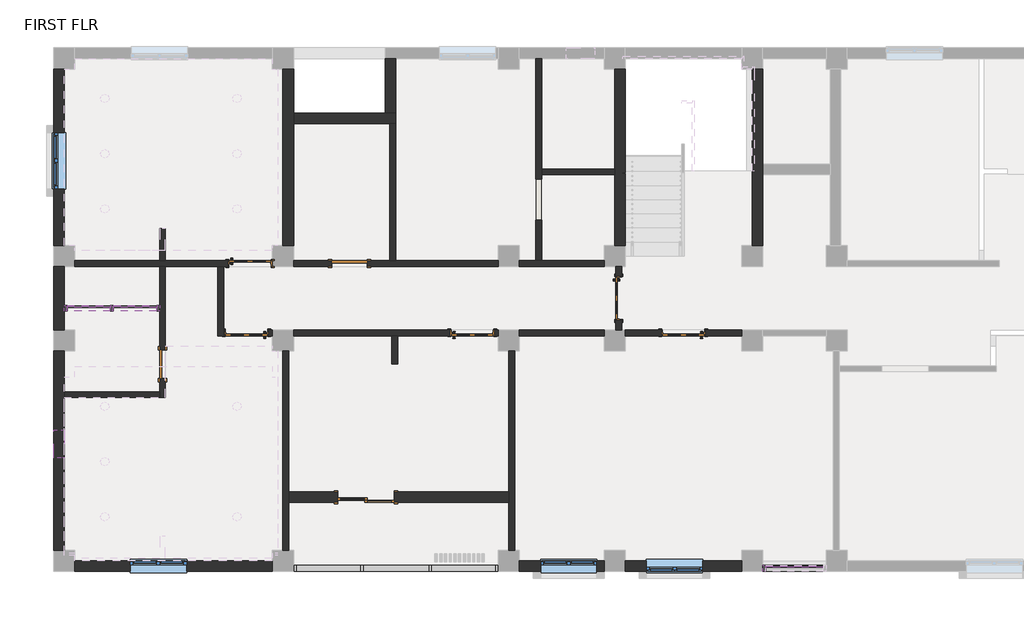
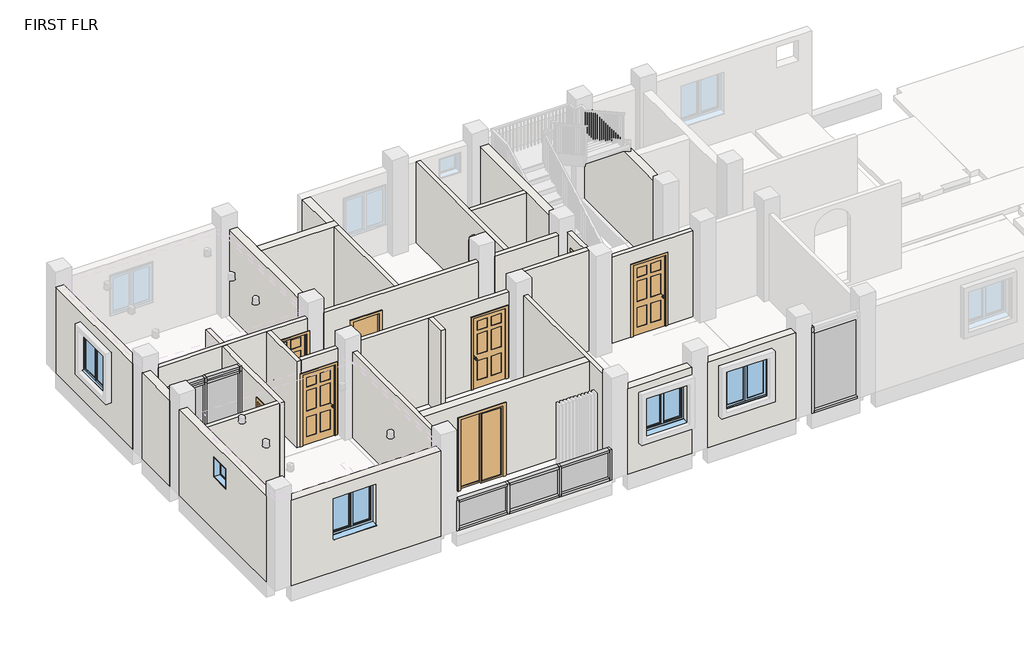
# One storey, part 1 of 5: 29 walls, 25 members, 9 plates, 8 doors, 5 windows.
"""IFC4 building model written with IfcOpenShell, lengths in millimetres."""

from ifc_helpers import new_model, si_unit, point, frame, origin, place, context, project, spatial, polyline, ellipse_curve, trimmed, outline, extrude, faceted_brep, transform, mapped, element, save
from ifc_brep_helpers import plane_surface, extruded_surface, advanced_brep
from components import door_double_sliding_4436dcad, door_c610b25b, door_03e3dfb5, single_flush_2_x_7_bath_room_door_025d1c86, door_e00f436c, member_f0fea5a5, member_f6f0dfdd, member_ee409385, member_876f8f00, member_2b4cd6f1, member_0dc43c0c, member_51239652, member_c58de4df, member_410c6227, member_73c23c35, member_71eb4692, system_panel_glazed_e8343dfa, system_panel_glazed_58efc156, system_panel_glazed_69a0d9e9, system_panel_glazed_27716cba, system_panel_glazed_e6f1e35b, system_panel_glazed_aa2ae1c5, window_80340324, w2_0001_4_x_4_window_9dec5fc7

model = new_model("IFC4")

# Units and contexts
model_context = context("Model", 3, world=origin())
ifc_project = project(units=[si_unit("LENGTHUNIT", "METRE", prefix="MILLI")], contexts=[model_context])

# Site, building, storey
site = spatial("IfcSite", under=ifc_project)
building = spatial("IfcBuilding", under=site)
storey = spatial("IfcBuildingStorey", under=building, Name="FIRST FLR", Elevation=3352.8)

# Doors
placement = place(None, origin())
door_double_sliding_shape = door_double_sliding_4436dcad(model_context)
element("IfcDoor", 1, ObjectType="Door-Double-Sliding", at=placement, inside=storey, context=model_context, shape_type="MappedRepresentation", body=[
    mapped(door_double_sliding_shape, transform((-8630.2456086, -9389.2679047, 3352.8), x_axis=(-1.0, 0.0, 0.0), y_axis=(0.0, -1.0, 0.0), z_axis=(0.0, 0.0, 1.0))),
])
door_shape = door_c610b25b(model_context)
element("IfcDoor", 2, ObjectType="Door-Interior-Single-6_Panel-Wood : 36\" x 84\"", at=placement, inside=storey, context=model_context, shape_type="MappedRepresentation", body=[
    mapped(door_shape, transform((-6331.5456086, -5967.8544704, 3352.8), x_axis=(1.0, 0.0, 0.0), y_axis=(0.0, 1.0, 0.0), z_axis=(0.0, 0.0, 1.0))),
])
element("IfcDoor", 3, ObjectType="Door-Interior-Single-6_Panel-Wood : 36\" x 84\"", at=placement, inside=storey, context=model_context, shape_type="MappedRepresentation", body=[
    mapped(door_shape, transform((-3172.4206086, -5215.3794704, 3352.8), x_axis=(0.0, -1.0, 0.0), y_axis=(1.0, 0.0, 0.0), z_axis=(0.0, 0.0, 1.0))),
])
door_2_shape = door_03e3dfb5(model_context)
element("IfcDoor", 4, ObjectType="Door-Interior-Single-6_Panel-Wood : 36\" x 84\"", at=placement, inside=storey, context=model_context, shape_type="MappedRepresentation", body=[
    mapped(door_2_shape, transform((-11207.742897, -5967.8544704, 3352.8), x_axis=(-1.0, 0.0, 0.0), y_axis=(0.0, -1.0, 0.0), z_axis=(0.0, 0.0, 1.0))),
])
element("IfcDoor", 5, ObjectType="Door-Interior-Single-6_Panel-Wood : 36\" x 84\"", at=placement, inside=storey, context=model_context, shape_type="MappedRepresentation", body=[
    mapped(door_2_shape, transform((-11132.1456086, -4462.9044704, 3352.8), x_axis=(1.0, 0.0, 0.0), y_axis=(0.0, 1.0, 0.0), z_axis=(0.0, 0.0, 1.0))),
])
element("IfcDoor", 6, ObjectType="Door-Interior-Single-6_Panel-Wood : 36\" x 84\"", at=placement, inside=storey, context=model_context, shape_type="MappedRepresentation", body=[
    mapped(door_2_shape, transform((-1773.9769742, -5967.8544704, 3352.8), x_axis=(-1.0, 0.0, 0.0), y_axis=(0.0, -1.0, 0.0), z_axis=(0.0, 0.0, 1.0))),
])
single_flush_2_x_7_bath_room_door_shape = single_flush_2_x_7_bath_room_door_025d1c86(model_context)
element("IfcDoor", 7, ObjectType="Single-Flush : 2' X 7' BATH ROOM DOOR", at=placement, inside=storey, context=model_context, shape_type="MappedRepresentation", body=[
    mapped(single_flush_2_x_7_bath_room_door_shape, transform((-13023.2401855, -6639.2659448, 3352.8), x_axis=(0.0, 1.0, 0.0), y_axis=(-1.0, 0.0, 0.0), z_axis=(0.0, 0.0, 1.0))),
])
door_3_shape = door_e00f436c(model_context)
element("IfcDoor", 8, ObjectType="Single-Flush : bathroom 2'6\" door", at=placement, inside=storey, context=model_context, shape_type="MappedRepresentation", body=[
    mapped(door_3_shape, transform((-8985.8456086, -4466.0794704, 3352.8), x_axis=(-1.0, 0.0, 0.0), y_axis=(0.0, -1.0, 0.0), z_axis=(0.0, 0.0, 1.0))),
])

# Members
member_shape = member_f0fea5a5(model_context)
element("IfcMember", 9, ObjectType="Rectangular Mullion : 2.5\" x 5\" rectangular", at=placement, inside=storey, context=model_context, shape_type="MappedRepresentation", body=[
    mapped(member_shape, transform((-14116.042897, -5431.2794704, 3352.8), x_axis=(1.0, 0.0, 0.0), y_axis=(0.0, -1.0, 0.0), z_axis=(0.0, 0.0, -1.0))),
])
member_2_shape = member_f6f0dfdd(model_context)
element("IfcMember", 10, ObjectType="Rectangular Mullion : 2.5\" x 5\" rectangular", at=placement, inside=storey, context=model_context, shape_type="MappedRepresentation", body=[
    mapped(member_2_shape, transform((-14116.042897, -5431.2794704, 5791.2), x_axis=(1.0, 0.0, 0.0), y_axis=(0.0, -1.0, 0.0), z_axis=(0.0, 0.0, -1.0))),
])
member_3_shape = member_ee409385(model_context)
element("IfcMember", 11, ObjectType="Rectangular Mullion : 2.5\" x 5\" rectangular", at=placement, inside=storey, context=model_context, shape_type="MappedRepresentation", body=[
    mapped(member_3_shape, transform((-13086.7401855, -5431.2794704, 3352.8), x_axis=(1.0, 0.0, 0.0), y_axis=(0.0, -1.0, 0.0), z_axis=(0.0, 0.0, -1.0))),
])
member_4_shape = member_876f8f00(model_context)
element("IfcMember", 12, ObjectType="Rectangular Mullion : 2.5\" x 5\" rectangular", at=placement, inside=storey, context=model_context, shape_type="MappedRepresentation", body=[
    mapped(member_4_shape, transform((-15145.3456086, -5431.2794704, 5943.6), x_axis=(-1.0, 0.0, 0.0), y_axis=(0.0, -1.0, 0.0), z_axis=(0.0, 0.0, 1.0))),
])
element("IfcMember", 13, ObjectType="Rectangular Mullion : 2.5\" x 5\" rectangular", at=placement, inside=storey, context=model_context, shape_type="MappedRepresentation", body=[
    mapped(member_4_shape, transform((-61.2083398, -11052.9679047, 5943.6), x_axis=(-1.0, 0.0, 0.0), y_axis=(0.0, -1.0, 0.0), z_axis=(0.0, 0.0, 1.0))),
])
element("IfcMember", 14, ObjectType="Rectangular Mullion : 2.5\" x 5\" rectangular", at=placement, inside=storey, context=model_context, shape_type="MappedRepresentation", body=[
    mapped(member_4_shape, transform((-13086.7401855, -5431.2794704, 5791.2), x_axis=(1.0, 0.0, 0.0), y_axis=(0.0, -1.0, 0.0), z_axis=(0.0, 0.0, -1.0))),
])
element("IfcMember", 15, ObjectType="Rectangular Mullion : 2.5\" x 5\" rectangular", at=placement, inside=storey, context=model_context, shape_type="MappedRepresentation", body=[
    mapped(member_3_shape, transform((-15145.3456086, -5431.2794704, 5791.2), x_axis=(-1.0, 0.0, 0.0), y_axis=(0.0, -1.0, 0.0), z_axis=(0.0, 0.0, 1.0))),
])
element("IfcMember", 16, ObjectType="Rectangular Mullion : 2.5\" x 5\" rectangular", at=placement, inside=storey, context=model_context, shape_type="MappedRepresentation", body=[
    mapped(member_3_shape, transform((-61.2083398, -11052.9679047, 5791.2), x_axis=(-1.0, 0.0, 0.0), y_axis=(0.0, -1.0, 0.0), z_axis=(0.0, 0.0, 1.0))),
])
member_5_shape = member_2b4cd6f1(model_context)
element("IfcMember", 17, ObjectType="Rectangular Mullion : 2.5\" x 5\" rectangular", at=placement, inside=storey, context=model_context, shape_type="MappedRepresentation", body=[
    mapped(member_5_shape, transform((-5836.2456086, -11052.9679047, 4267.2), x_axis=(0.0, 0.0, 1.0), y_axis=(0.0, -1.0, 0.0), z_axis=(1.0, 0.0, 0.0))),
])
element("IfcMember", 18, ObjectType="Rectangular Mullion : 2.5\" x 5\" rectangular", at=placement, inside=storey, context=model_context, shape_type="MappedRepresentation", body=[
    mapped(member_5_shape, transform((-8750.8956085, -11052.9679047, 4267.2), x_axis=(0.0, 0.0, 1.0), y_axis=(0.0, -1.0, 0.0), z_axis=(1.0, 0.0, 0.0))),
])
element("IfcMember", 19, ObjectType="Rectangular Mullion : 2.5\" x 5\" rectangular", at=placement, inside=storey, context=model_context, shape_type="MappedRepresentation", body=[
    mapped(member_5_shape, transform((-10128.8456086, -11052.9679047, 3352.8), x_axis=(0.0, 0.0, -1.0), y_axis=(0.0, -1.0, 0.0), z_axis=(-1.0, 0.0, 0.0))),
])
element("IfcMember", 20, ObjectType="Rectangular Mullion : 2.5\" x 5\" rectangular", at=placement, inside=storey, context=model_context, shape_type="MappedRepresentation", body=[
    mapped(member_5_shape, transform((-7214.1956087, -11052.9679047, 3352.8), x_axis=(0.0, 0.0, -1.0), y_axis=(0.0, -1.0, 0.0), z_axis=(-1.0, 0.0, 0.0))),
])
member_6_shape = member_0dc43c0c(model_context)
element("IfcMember", 21, ObjectType="Rectangular Mullion : 2.5\" x 5\" rectangular", at=placement, inside=storey, context=model_context, shape_type="MappedRepresentation", body=[
    mapped(member_6_shape, transform((-7277.6956087, -11052.9679047, 4267.2), x_axis=(0.0, 0.0, 1.0), y_axis=(0.0, -1.0, 0.0), z_axis=(1.0, 0.0, 0.0))),
])
element("IfcMember", 22, ObjectType="Rectangular Mullion : 2.5\" x 5\" rectangular", at=placement, inside=storey, context=model_context, shape_type="MappedRepresentation", body=[
    mapped(member_6_shape, transform((-8687.3956085, -11052.9679047, 3352.8), x_axis=(0.0, 0.0, -1.0), y_axis=(0.0, -1.0, 0.0), z_axis=(-1.0, 0.0, 0.0))),
])
member_7_shape = member_51239652(model_context)
element("IfcMember", 23, ObjectType="Rectangular Mullion : 2.5\" x 5\" rectangular", at=placement, inside=storey, context=model_context, shape_type="MappedRepresentation", body=[
    mapped(member_7_shape, transform((-13150.2401855, -5431.2794704, 5943.6), x_axis=(0.0, 0.0, 1.0), y_axis=(0.0, -1.0, 0.0), z_axis=(1.0, 0.0, 0.0))),
])
element("IfcMember", 24, ObjectType="Rectangular Mullion : 2.5\" x 5\" rectangular", at=placement, inside=storey, context=model_context, shape_type="MappedRepresentation", body=[
    mapped(member_7_shape, transform((-14147.792897, -5431.2794704, 5943.6), x_axis=(0.0, 0.0, 1.0), y_axis=(0.0, -1.0, 0.0), z_axis=(1.0, 0.0, 0.0))),
])
element("IfcMember", 25, ObjectType="Rectangular Mullion : 2.5\" x 5\" rectangular", at=placement, inside=storey, context=model_context, shape_type="MappedRepresentation", body=[
    mapped(member_7_shape, transform((-15081.8456086, -5431.2794704, 3352.8), x_axis=(0.0, 0.0, -1.0), y_axis=(0.0, -1.0, 0.0), z_axis=(-1.0, 0.0, 0.0))),
])
element("IfcMember", 26, ObjectType="Rectangular Mullion : 2.5\" x 5\" rectangular", at=placement, inside=storey, context=model_context, shape_type="MappedRepresentation", body=[
    mapped(member_7_shape, transform((-14084.292897, -5431.2794704, 3352.8), x_axis=(0.0, 0.0, -1.0), y_axis=(0.0, -1.0, 0.0), z_axis=(-1.0, 0.0, 0.0))),
])
member_8_shape = member_c58de4df(model_context)
element("IfcMember", 27, ObjectType="Rectangular Mullion : 2.5\" x 5\" rectangular", at=placement, inside=storey, context=model_context, shape_type="MappedRepresentation", body=[
    mapped(member_8_shape, transform((-14147.792897, -5431.2794704, 5791.2), x_axis=(0.0, 0.0, 1.0), y_axis=(0.0, -1.0, 0.0), z_axis=(1.0, 0.0, 0.0))),
])
element("IfcMember", 28, ObjectType="Rectangular Mullion : 2.5\" x 5\" rectangular", at=placement, inside=storey, context=model_context, shape_type="MappedRepresentation", body=[
    mapped(member_8_shape, transform((-13150.2401855, -5431.2794704, 5791.2), x_axis=(0.0, 0.0, 1.0), y_axis=(0.0, -1.0, 0.0), z_axis=(1.0, 0.0, 0.0))),
])
member_9_shape = member_410c6227(model_context)
element("IfcMember", 29, ObjectType="Rectangular Mullion : 2.5\" x 5\" rectangular", at=placement, inside=storey, context=model_context, shape_type="MappedRepresentation", body=[
    mapped(member_9_shape, transform((-8719.1456085, -11052.9679047, 3352.8), x_axis=(1.0, 0.0, 0.0), y_axis=(0.0, -1.0, 0.0), z_axis=(0.0, 0.0, -1.0))),
])
element("IfcMember", 30, ObjectType="Rectangular Mullion : 2.5\" x 5\" rectangular", at=placement, inside=storey, context=model_context, shape_type="MappedRepresentation", body=[
    mapped(member_9_shape, transform((-7245.9456087, -11052.9679047, 3352.8), x_axis=(1.0, 0.0, 0.0), y_axis=(0.0, -1.0, 0.0), z_axis=(0.0, 0.0, -1.0))),
])
member_10_shape = member_73c23c35(model_context)
element("IfcMember", 31, ObjectType="Rectangular Mullion : 2.5\" x 5\" rectangular", at=placement, inside=storey, context=model_context, shape_type="MappedRepresentation", body=[
    mapped(member_10_shape, transform((-5772.7456086, -11052.9679047, 3352.8), x_axis=(1.0, 0.0, 0.0), y_axis=(0.0, -1.0, 0.0), z_axis=(0.0, 0.0, -1.0))),
])
element("IfcMember", 32, ObjectType="Rectangular Mullion : 2.5\" x 5\" rectangular", at=placement, inside=storey, context=model_context, shape_type="MappedRepresentation", body=[
    mapped(member_10_shape, transform((-10192.3456086, -11052.9679047, 4267.2), x_axis=(-1.0, 0.0, 0.0), y_axis=(0.0, -1.0, 0.0), z_axis=(0.0, 0.0, 1.0))),
])
member_11_shape = member_71eb4692(model_context)
element("IfcMember", 33, ObjectType="Rectangular Mullion : 2.5\" x 5\" rectangular", at=placement, inside=storey, context=model_context, shape_type="MappedRepresentation", body=[
    mapped(member_11_shape, transform((2.2916602, -11052.9679047, 3352.8), x_axis=(0.0, 0.0, -1.0), y_axis=(0.0, -1.0, 0.0), z_axis=(-1.0, 0.0, 0.0))),
])

# Plates
system_panel_glazed_shape = system_panel_glazed_e8343dfa(model_context)
element("IfcPlate", 34, ObjectType="System Panel : Glazed", at=placement, inside=storey, context=model_context, shape_type="MappedRepresentation", body=[
    mapped(system_panel_glazed_shape, transform((-14614.8192528, -5431.2794704, 3416.3), x_axis=(1.0, 0.0, 0.0), y_axis=(0.0, 1.0, 0.0), z_axis=(0.0, 0.0, 1.0))),
])
element("IfcPlate", 35, ObjectType="System Panel : Glazed", at=placement, inside=storey, context=model_context, shape_type="MappedRepresentation", body=[
    mapped(system_panel_glazed_shape, transform((-13617.2665413, -5431.2794704, 3416.3), x_axis=(1.0, 0.0, 0.0), y_axis=(0.0, 1.0, 0.0), z_axis=(0.0, 0.0, 1.0))),
])
system_panel_glazed_2_shape = system_panel_glazed_58efc156(model_context)
element("IfcPlate", 36, ObjectType="System Panel : Glazed", at=placement, inside=storey, context=model_context, shape_type="MappedRepresentation", body=[
    mapped(system_panel_glazed_2_shape, transform((-14614.8192528, -5431.2794704, 5822.95), x_axis=(1.0, 0.0, 0.0), y_axis=(0.0, 1.0, 0.0), z_axis=(0.0, 0.0, 1.0))),
])
element("IfcPlate", 37, ObjectType="System Panel : Glazed", at=placement, inside=storey, context=model_context, shape_type="MappedRepresentation", body=[
    mapped(system_panel_glazed_2_shape, transform((-13617.2665413, -5431.2794704, 5822.95), x_axis=(1.0, 0.0, 0.0), y_axis=(0.0, 1.0, 0.0), z_axis=(0.0, 0.0, 1.0))),
])
system_panel_glazed_3_shape = system_panel_glazed_69a0d9e9(model_context)
element("IfcPlate", 38, ObjectType="System Panel : Glazed", at=placement, inside=storey, context=model_context, shape_type="MappedRepresentation", body=[
    mapped(system_panel_glazed_3_shape, transform((-9439.8706086, -11052.9679047, 3416.3), x_axis=(1.0, 0.0, 0.0), y_axis=(0.0, 1.0, 0.0), z_axis=(0.0, 0.0, 1.0))),
])
element("IfcPlate", 39, ObjectType="System Panel : Glazed", at=placement, inside=storey, context=model_context, shape_type="MappedRepresentation", body=[
    mapped(system_panel_glazed_3_shape, transform((-6525.2206087, -11052.9679047, 3416.3), x_axis=(1.0, 0.0, 0.0), y_axis=(0.0, 1.0, 0.0), z_axis=(0.0, 0.0, 1.0))),
])
system_panel_glazed_4_shape = system_panel_glazed_27716cba(model_context)
element("IfcPlate", 40, ObjectType="System Panel : Glazed", at=placement, inside=storey, context=model_context, shape_type="MappedRepresentation", body=[
    mapped(system_panel_glazed_4_shape, transform((-7982.5456086, -11052.9679047, 3416.3), x_axis=(1.0, 0.0, 0.0), y_axis=(0.0, 1.0, 0.0), z_axis=(0.0, 0.0, 1.0))),
])
system_panel_glazed_5_shape = system_panel_glazed_e6f1e35b(model_context)
element("IfcPlate", 41, ObjectType="System Panel : Glazed", at=placement, inside=storey, context=model_context, shape_type="MappedRepresentation", body=[
    mapped(system_panel_glazed_5_shape, transform((624.5916602, -11052.9679047, 3416.3), x_axis=(1.0, 0.0, 0.0), y_axis=(0.0, 1.0, 0.0), z_axis=(0.0, 0.0, 1.0))),
])
system_panel_glazed_6_shape = system_panel_glazed_aa2ae1c5(model_context)
element("IfcPlate", 42, ObjectType="System Panel : Glazed", at=placement, inside=storey, context=model_context, shape_type="MappedRepresentation", body=[
    mapped(system_panel_glazed_6_shape, transform((624.5916602, -11052.9679047, 5822.95), x_axis=(1.0, 0.0, 0.0), y_axis=(0.0, 1.0, 0.0), z_axis=(0.0, 0.0, 1.0))),
])

# Walls
element("IfcWall", 43, ObjectType="EXTERIOR WALL 9\"", at=placement, inside=storey, context=model_context, shape_type="SweptSolid", body=[
    extrude(outline(polyline([(3352.8, -14916.7456086), (3352.8, -10649.5456086), (5943.6, -10649.5456086), (5943.6, -14916.7456086), (3352.8, -14916.7456086)]), holes=[polyline([(4352.8, -12503.7456086), (4352.8, -13722.9456086), (5572.0, -13722.9456086), (5572.0, -12503.7456086), (4352.8, -12503.7456086)])]), frame((0.0, -11116.4679047, 0.0), z_axis=(0.0, 1.0, 0.0), x_axis=(0.0, 0.0, 1.0)), (0.0, 0.0, 1.0), 228.6),
])
element("IfcWall", 44, ObjectType="EXTERIOR WALL 9\"", at=placement, inside=storey, context=model_context, shape_type="SweptSolid", body=[
    extrude(outline(polyline([(3352.8, -5315.5456086), (3352.8, -3486.7456086), (5943.6, -3486.7456086), (5943.6, -5315.5456086), (3352.8, -5315.5456086)]), holes=[polyline([(4352.8, -3639.1456086), (4352.8, -4858.3456086), (5572.0, -4858.3456086), (5572.0, -3639.1456086), (4352.8, -3639.1456086)])]), frame((0.0, -11116.4679047, 0.0), z_axis=(0.0, 1.0, 0.0), x_axis=(0.0, 0.0, 1.0)), (0.0, 0.0, 1.0), 228.6),
])
element("IfcWall", 45, ObjectType="EXTERIOR WALL 9\"", at=placement, inside=storey, context=model_context, shape_type="SweptSolid", body=[
    extrude(outline(polyline([(3352.8, -3029.5456086), (3352.8, -518.4083398), (5943.6, -518.4083398), (5943.6, -3029.5456086), (3352.8, -3029.5456086)]), holes=[polyline([(4352.8, -2572.3456086), (5572.0, -2572.3456086), (5572.0, -1353.1456086), (4352.8, -1353.1456086), (4352.8, -2572.3456086)])]), frame((0.0, -11116.4679047, 0.0), z_axis=(0.0, 1.0, 0.0), x_axis=(0.0, 0.0, 1.0)), (0.0, 0.0, 1.0), 228.6),
])
element("IfcWall", 46, ObjectType="EXTERIOR WALL 9\"", at=placement, inside=storey, context=model_context, shape_type="Brep", body=[
    faceted_brep([(-15145.3456086, -10659.2679047, 3352.8), (-15145.3456086, -7363.1659448, 3352.8), (-15145.3456086, -7236.1659448, 3352.8), (-15145.3456086, -6358.3794704, 3352.8), (-15145.3456086, -6358.3794704, 5943.6), (-15145.3456086, -7236.1659448, 5943.6), (-15145.3456086, -7363.1659448, 5943.6), (-15145.3456086, -10659.2679047, 5943.6), (-15145.3456086, -8671.2659448, 5559.8263913), (-15145.3456086, -8061.6659448, 5559.8263913), (-15145.3456086, -8061.6659448, 4950.2263913), (-15145.3456086, -8671.2659448, 4950.2263913), (-15373.9456086, -10659.2679047, 3352.8), (-15373.9456086, -10659.2679047, 5943.6), (-15373.9456086, -6358.3794704, 5943.6), (-15373.9456086, -6358.3794704, 3352.8), (-15373.9456086, -8671.2659448, 5559.8263913), (-15373.9456086, -8671.2659448, 4950.2263913), (-15373.9456086, -8061.6659448, 4950.2263913), (-15373.9456086, -8061.6659448, 5559.8263913)], [[[0, 1, 2, 3, 4, 5, 6, 7], [8, 9, 10, 11]], [[12, 13, 14, 15], [16, 17, 18, 19]], [[3, 2, 1, 0, 12, 15]], [[4, 3, 15, 14]], [[7, 6, 5, 4, 14, 13]], [[0, 7, 13, 12]], [[17, 16, 8, 11]], [[18, 17, 11, 10]], [[19, 18, 10, 9]], [[16, 19, 9, 8]]]),
])
element("IfcWall", 47, ObjectType="EXTERIOR WALL 9\"", at=placement, inside=storey, context=model_context, shape_type="Brep", body=[
    faceted_brep([(-15145.3456086, -5901.1794704, 3352.8), (-15145.3456086, -5431.2794704, 3352.8), (-15145.3456086, -5304.2794704, 3352.8), (-15145.3456086, -4529.5794704, 3352.8), (-15145.3456086, -4529.5794704, 5943.6), (-15145.3456086, -5304.2794704, 5943.6), (-15145.3456086, -5431.2794704, 5943.6), (-15145.3456086, -5901.1794704, 5943.6), (-15373.9456086, -5901.1794704, 3352.8), (-15373.9456086, -5901.1794704, 5943.6), (-15373.9456086, -4529.5794704, 5943.6), (-15373.9456086, -4529.5794704, 3352.8)], [[[0, 1, 2, 3, 4, 5, 6, 7]], [[8, 9, 10, 11]], [[3, 2, 1, 0, 8, 11]], [[4, 3, 11, 10]], [[7, 6, 5, 4, 10, 9]], [[0, 7, 9, 8]]]),
])
element("IfcWall", 48, ObjectType="EXTERIOR WALL 9\"", at=placement, inside=storey, context=model_context, shape_type="SweptSolid", body=[
    extrude(outline(polyline([(-4072.3794704, 3352.8), (-4072.3794704, 5943.6), (-262.3794704, 5943.6), (-262.3794704, 3352.8), (-4072.3794704, 3352.8)]), holes=[polyline([(-1633.9794704, 4267.2), (-1633.9794704, 5486.4), (-2853.1794704, 5486.4), (-2853.1794704, 4267.2), (-1633.9794704, 4267.2)])]), frame((-15373.9456086, 0.0, 0.0), z_axis=(1.0, 0.0, 0.0), x_axis=(0.0, 1.0, 0.0)), (0.0, 0.0, 1.0), 228.6),
])
element("IfcWall", 49, ObjectType="EXTERIOR WALL 9\"", at=placement, inside=storey, context=model_context, shape_type="Brep", body=[
    faceted_brep([(-10420.9456086, -262.3794704, 3352.8), (-10420.9456086, -4072.3794704, 3352.8), (-10420.9456086, -4072.3794704, 5943.6), (-10420.9456086, -262.3794704, 5943.6), (-10192.3456086, -262.3794704, 3352.8), (-10192.3456086, -262.3794704, 5943.6), (-10192.3456086, -1214.8794704, 5943.6), (-10192.3456086, -1443.4794704, 5943.6), (-10192.3456086, -4072.3794704, 5943.6), (-10192.3456086, -4072.3794704, 3352.8), (-10192.3456086, -1443.4794704, 3352.8), (-10192.3456086, -1214.8794704, 3352.8)], [[[0, 1, 2, 3]], [[4, 5, 6, 7, 8, 9, 10, 11]], [[1, 0, 4, 11, 10, 9]], [[2, 1, 9, 8]], [[3, 2, 8, 7, 6, 5]], [[0, 3, 5, 4]]]),
])
element("IfcWall", 50, ObjectType="EXTERIOR WALL 9\"", at=placement, inside=storey, context=model_context, shape_type="SweptSolid", body=[
    extrude(outline(polyline([(3352.8, -10293.9456086), (3352.8, -9239.8456086), (5486.4, -9239.8456086), (5486.4, -8020.6456086), (3352.8, -8020.6456086), (3352.8, -5544.1456086), (5943.6, -5544.1456086), (5943.6, -10293.9456086), (3352.8, -10293.9456086)])), frame((0.0, -9630.5679047, 0.0), z_axis=(0.0, 1.0, 0.0), x_axis=(0.0, 0.0, 1.0)), (0.0, 0.0, 1.0), 228.6),
])
element("IfcWall", 51, ObjectType="EXTERIOR WALL 9\"", at=placement, inside=storey, context=model_context, shape_type="Brep", body=[
    faceted_brep([(-10192.3456086, -1443.4794704, 3352.8), (-8109.5456086, -1443.4794704, 3352.8), (-7982.5456086, -1443.4794704, 3352.8), (-7982.5456086, -1443.4794704, 5943.6), (-8109.5456086, -1443.4794704, 5943.6), (-10192.3456086, -1443.4794704, 5943.6), (-10192.3456086, -1214.8794704, 3352.8), (-10192.3456086, -1214.8794704, 5943.6), (-8211.1456086, -1214.8794704, 5943.6), (-7982.5456086, -1214.8794704, 5943.6), (-7982.5456086, -1214.8794704, 3352.8), (-8211.1456086, -1214.8794704, 3352.8)], [[[0, 1, 2, 3, 4, 5]], [[6, 7, 8, 9, 10, 11]], [[2, 1, 0, 6, 11, 10]], [[5, 4, 3, 9, 8, 7]], [[0, 5, 7, 6]], [[3, 2, 10, 9]]]),
])
element("IfcWall", 52, ObjectType="EXTERIOR WALL 9\"", at=placement, inside=storey, context=model_context, shape_type="SweptSolid", body=[
    extrude(outline(polyline([(-7982.5456086, -33.7794704), (-7982.5456086, -1214.8794704), (-8211.1456086, -1214.8794704), (-8211.1456086, -33.7794704), (-7982.5456086, -33.7794704)])), frame((0.0, 0.0, 3352.8), z_axis=(0.0, 0.0, 1.0), x_axis=(1.0, 0.0, 0.0)), (0.0, 0.0, 1.0), 2590.8),
])
element("IfcWall", 53, ObjectType="EXTERIOR WALL 9\"", at=placement, inside=storey, context=model_context, shape_type="Brep", body=[
    faceted_brep([(-3258.1456086, -262.3794704, 3352.8), (-3258.1456086, -2421.3794704, 3352.8), (-3258.1456086, -2548.3794704, 3352.8), (-3258.1456086, -4072.3794704, 3352.8), (-3258.1456086, -4072.3794704, 5943.6), (-3258.1456086, -2548.3794704, 5943.6), (-3258.1456086, -2421.3794704, 5943.6), (-3258.1456086, -262.3794704, 5943.6), (-3029.5456086, -262.3794704, 3352.8), (-3029.5456086, -262.3794704, 5943.6), (-3029.5456086, -4072.3794704, 5943.6), (-3029.5456086, -4072.3794704, 3352.8)], [[[0, 1, 2, 3, 4, 5, 6, 7]], [[8, 9, 10, 11]], [[3, 2, 1, 0, 8, 11]], [[4, 3, 11, 10]], [[7, 6, 5, 4, 10, 9]], [[0, 7, 9, 8]]]),
])
element("IfcWall", 54, ObjectType="EXTERIOR WALL 9\"", at=placement, inside=storey, context=model_context, shape_type="Brep", body=[
    faceted_brep([(-289.8083398, -262.3794704, 3352.8), (-289.8083398, -4072.3794704, 3352.8), (-289.8083398, -4072.3794704, 5943.6), (-289.8083398, -262.3794704, 5943.6), (-61.2083398, -262.3794704, 3352.8), (-61.2083398, -262.3794704, 5943.6), (-61.2083398, -2319.7794704, 5943.6), (-61.2083398, -2548.3794704, 5943.6), (-61.2083398, -4072.3794704, 5943.6), (-61.2083398, -4072.3794704, 3352.8), (-61.2083398, -2548.3794704, 3352.8), (-61.2083398, -2319.7794704, 3352.8)], [[[0, 1, 2, 3]], [[4, 5, 6, 7, 8, 9, 10, 11]], [[1, 0, 4, 11, 10, 9]], [[2, 1, 9, 8]], [[3, 2, 8, 7, 6, 5]], [[0, 3, 5, 4]]]),
])
element("IfcWall", 55, ObjectType="INTERIOR WALL 5\"", at=placement, inside=storey, context=model_context, shape_type="Brep", body=[
    faceted_brep([(-10649.5456086, -4529.5794704, 5943.6), (-11702.4401855, -4529.5794704, 5943.6), (-11829.4401855, -4529.5794704, 5943.6), (-12959.7401855, -4529.5794704, 5943.6), (-13086.7401855, -4529.5794704, 5943.6), (-14916.7456086, -4529.5794704, 5943.6), (-14916.7456086, -4529.5794704, 3352.8), (-13086.7401855, -4529.5794704, 3352.8), (-12959.7401855, -4529.5794704, 3352.8), (-11829.4401855, -4529.5794704, 3352.8), (-11702.4401855, -4529.5794704, 3352.8), (-11614.7456086, -4529.5794704, 3352.8), (-11614.7456086, -4529.5794704, 5511.8), (-10649.5456086, -4529.5794704, 5511.8), (-14916.7456086, -4402.5794704, 5943.6), (-13086.7401855, -4402.5794704, 5943.6), (-12959.7401855, -4402.5794704, 5943.6), (-10649.5456086, -4402.5794704, 5943.6), (-10649.5456086, -4402.5794704, 5511.8), (-11614.7456086, -4402.5794704, 5511.8), (-11614.7456086, -4402.5794704, 3352.8), (-12959.7401855, -4402.5794704, 3352.8), (-13086.7401855, -4402.5794704, 3352.8), (-14916.7456086, -4402.5794704, 3352.8)], [[[0, 1, 2, 3, 4, 5, 6, 7, 8, 9, 10, 11, 12, 13]], [[14, 15, 16, 17, 18, 19, 20, 21, 22, 23]], [[6, 23, 22, 21, 20, 11, 10, 9, 8, 7]], [[17, 0, 13, 18]], [[5, 4, 3, 2, 1, 0, 17, 16, 15, 14]], [[6, 5, 14, 23]], [[12, 19, 18, 13]], [[19, 12, 11, 20]]]),
])
element("IfcWall", 56, ObjectType="INTERIOR WALL 5\"", at=placement, inside=storey, context=model_context, shape_type="Brep", body=[
    faceted_brep([(-13086.7401855, -3705.5659448, 5943.6), (-13086.7401855, -3705.5659448, 3352.8), (-13086.7401855, -4402.5794704, 3352.8), (-13086.7401855, -4402.5794704, 5943.6), (-12959.7401855, -3705.5659448, 3352.8), (-12959.7401855, -3705.5659448, 5943.6), (-12959.7401855, -4402.5794704, 5943.6), (-12959.7401855, -4402.5794704, 3352.8)], [[[0, 1, 2, 3]], [[4, 5, 6, 7]], [[1, 4, 7, 2]], [[5, 0, 3, 6]], [[1, 0, 5, 4]], [[3, 2, 7, 6]]]),
    faceted_brep([(-13086.7401855, -7363.1659448, 3352.8), (-13086.7401855, -7363.1659448, 5943.6), (-13086.7401855, -7236.1659448, 5943.6), (-13086.7401855, -5431.2794704, 5943.6), (-13086.7401855, -5304.2794704, 5943.6), (-13086.7401855, -4529.5794704, 5943.6), (-13086.7401855, -4529.5794704, 3352.8), (-13086.7401855, -5304.2794704, 3352.8), (-13086.7401855, -5431.2794704, 3352.8), (-13086.7401855, -6334.4659448, 3352.8), (-13086.7401855, -6334.4659448, 5384.8), (-13086.7401855, -6944.0659448, 5384.8), (-13086.7401855, -6944.0659448, 3352.8), (-13086.7401855, -7236.1659448, 3352.8), (-12959.7401855, -7363.1659448, 5943.6), (-12959.7401855, -7363.1659448, 3352.8), (-12959.7401855, -6944.0659448, 3352.8), (-12959.7401855, -6944.0659448, 5384.8), (-12959.7401855, -6334.4659448, 5384.8), (-12959.7401855, -6334.4659448, 3352.8), (-12959.7401855, -4529.5794704, 3352.8), (-12959.7401855, -4529.5794704, 5943.6)], [[[0, 1, 2, 3, 4, 5, 6, 7, 8, 9, 10, 11, 12, 13]], [[14, 15, 16, 17, 18, 19, 20, 21]], [[15, 0, 13, 12, 16]], [[19, 9, 8, 7, 6, 20]], [[1, 14, 21, 5, 4, 3, 2]], [[6, 5, 21, 20]], [[1, 0, 15, 14]], [[10, 9, 19, 18]], [[11, 10, 18, 17]], [[12, 11, 17, 16]]]),
])
element("IfcWall", 57, ObjectType="INTERIOR WALL 5\"", at=placement, inside=storey, context=model_context, shape_type="SweptSolid", body=[
    extrude(outline(polyline([(-15145.3456086, -7236.1659448), (-13086.7401855, -7236.1659448), (-13086.7401855, -7363.1659448), (-15145.3456086, -7363.1659448), (-15145.3456086, -7236.1659448)])), frame((0.0, 0.0, 3352.8), z_axis=(0.0, 0.0, 1.0), x_axis=(1.0, 0.0, 0.0)), (0.0, 0.0, 1.0), 2590.8),
])
element("IfcWall", 58, ObjectType="INTERIOR WALL 5\"", at=placement, inside=storey, context=model_context, shape_type="Brep", body=[
    faceted_brep([(-10293.9456086, -10659.2679047, 3352.8), (-10293.9456086, -9630.5679047, 3352.8), (-10293.9456086, -9401.9679047, 3352.8), (-10293.9456086, -6358.3794704, 3352.8), (-10293.9456086, -6358.3794704, 5943.6), (-10293.9456086, -9401.9679047, 5943.6), (-10293.9456086, -9630.5679047, 5943.6), (-10293.9456086, -10659.2679047, 5943.6), (-10420.9456086, -10659.2679047, 3352.8), (-10420.9456086, -10659.2679047, 5943.6), (-10420.9456086, -6358.3794704, 5943.6), (-10420.9456086, -6358.3794704, 3352.8)], [[[0, 1, 2, 3, 4, 5, 6, 7]], [[8, 9, 10, 11]], [[3, 2, 1, 0, 8, 11]], [[4, 3, 11, 10]], [[7, 6, 5, 4, 10, 9]], [[0, 7, 9, 8]]]),
])
element("IfcWall", 59, ObjectType="INTERIOR WALL 5\"", at=placement, inside=storey, context=model_context, shape_type="Brep", body=[
    faceted_brep([(-10192.3456086, -5901.1794704, 3352.8), (-10192.3456086, -5901.1794704, 5943.6), (-5772.7456086, -5901.1794704, 5943.6), (-5772.7456086, -5901.1794704, 3352.8), (-5848.9456086, -5901.1794704, 3352.8), (-5848.9456086, -5901.1794704, 5511.8), (-6814.1456086, -5901.1794704, 5511.8), (-6814.1456086, -5901.1794704, 3352.8), (-10192.3456086, -6028.1794704, 5943.6), (-10192.3456086, -6028.1794704, 3352.8), (-8071.4456086, -6028.1794704, 3352.8), (-7944.4456086, -6028.1794704, 3352.8), (-6814.1456086, -6028.1794704, 3352.8), (-6814.1456086, -6028.1794704, 5511.8), (-5848.9456086, -6028.1794704, 5511.8), (-5848.9456086, -6028.1794704, 3352.8), (-5772.7456086, -6028.1794704, 3352.8), (-5772.7456086, -6028.1794704, 5943.6), (-7944.4456086, -6028.1794704, 5943.6), (-8071.4456086, -6028.1794704, 5943.6)], [[[0, 1, 2, 3, 4, 5, 6, 7]], [[8, 9, 10, 11, 12, 13, 14, 15, 16, 17, 18, 19]], [[9, 0, 7, 12, 11, 10]], [[3, 16, 15, 4]], [[1, 0, 9, 8]], [[2, 1, 8, 19, 18, 17]], [[3, 2, 17, 16]], [[14, 5, 4, 15]], [[5, 14, 13, 6]], [[6, 13, 12, 7]]]),
])
element("IfcWall", 60, ObjectType="INTERIOR WALL 5\"", at=placement, inside=storey, context=model_context, shape_type="SweptSolid", body=[
    extrude(outline(polyline([(-8071.4456086, -6637.7794704), (-8071.4456086, -6028.1794704), (-7944.4456086, -6028.1794704), (-7944.4456086, -6637.7794704), (-8071.4456086, -6637.7794704)])), frame((0.0, 0.0, 3352.8), z_axis=(0.0, 0.0, 1.0), x_axis=(1.0, 0.0, 0.0)), (0.0, 0.0, 1.0), 2590.8),
])
element("IfcWall", 61, ObjectType="INTERIOR WALL 5\"", at=placement, inside=storey, context=model_context, shape_type="Brep", body=[
    faceted_brep([(-5417.1456086, -10659.2679047, 3352.8), (-5417.1456086, -6358.3794704, 3352.8), (-5417.1456086, -6358.3794704, 5943.6), (-5417.1456086, -10659.2679047, 5943.6), (-5544.1456086, -10659.2679047, 3352.8), (-5544.1456086, -10659.2679047, 5943.6), (-5544.1456086, -9630.5679047, 5943.6), (-5544.1456086, -9401.9679047, 5943.6), (-5544.1456086, -6358.3794704, 5943.6), (-5544.1456086, -6358.3794704, 3352.8), (-5544.1456086, -9401.9679047, 3352.8), (-5544.1456086, -9630.5679047, 3352.8)], [[[0, 1, 2, 3]], [[4, 5, 6, 7, 8, 9, 10, 11]], [[1, 0, 4, 11, 10, 9]], [[2, 1, 9, 8]], [[3, 2, 8, 7, 6, 5]], [[0, 3, 5, 4]]]),
])
element("IfcWall", 62, ObjectType="INTERIOR WALL 5\"", at=placement, inside=storey, context=model_context, shape_type="Brep", body=[
    faceted_brep([(-10192.3456086, -4529.5794704, 3352.8), (-9366.8456086, -4529.5794704, 3352.8), (-9366.8456086, -4529.5794704, 5384.8), (-8604.8456086, -4529.5794704, 5384.8), (-8604.8456086, -4529.5794704, 3352.8), (-5772.7456086, -4529.5794704, 3352.8), (-5772.7456086, -4529.5794704, 5943.6), (-10192.3456086, -4529.5794704, 5943.6), (-9366.8456086, -4402.5794704, 5384.8), (-9366.8456086, -4402.5794704, 3352.8), (-10192.3456086, -4402.5794704, 3352.8), (-10192.3456086, -4402.5794704, 5943.6), (-8109.5456086, -4402.5794704, 5943.6), (-7982.5456086, -4402.5794704, 5943.6), (-5772.7456086, -4402.5794704, 5943.6), (-5772.7456086, -4402.5794704, 3352.8), (-7982.5456086, -4402.5794704, 3352.8), (-8109.5456086, -4402.5794704, 3352.8), (-8604.8456086, -4402.5794704, 3352.8), (-8604.8456086, -4402.5794704, 5384.8)], [[[0, 1, 2, 3, 4, 5, 6, 7]], [[8, 9, 10, 11, 12, 13, 14, 15, 16, 17, 18, 19]], [[10, 9, 1, 0]], [[18, 17, 16, 15, 5, 4]], [[6, 5, 15, 14]], [[7, 6, 14, 13, 12, 11]], [[0, 7, 11, 10]], [[2, 1, 9, 8]], [[3, 2, 8, 19]], [[4, 3, 19, 18]]]),
])
element("IfcWall", 63, ObjectType="INTERIOR WALL 5\"", at=placement, inside=storey, context=model_context, shape_type="Brep", body=[
    faceted_brep([(-5315.5456086, -4529.5794704, 3352.8), (-3486.7456086, -4529.5794704, 3352.8), (-3486.7456086, -4529.5794704, 5943.6), (-5315.5456086, -4529.5794704, 5943.6), (-5315.5456086, -4402.5794704, 3352.8), (-5315.5456086, -4402.5794704, 5943.6), (-4959.9456086, -4402.5794704, 5943.6), (-4832.9456086, -4402.5794704, 5943.6), (-3486.7456086, -4402.5794704, 5943.6), (-3486.7456086, -4402.5794704, 3352.8), (-4832.9456086, -4402.5794704, 3352.8), (-4959.9456086, -4402.5794704, 3352.8)], [[[0, 1, 2, 3]], [[4, 5, 6, 7, 8, 9, 10, 11]], [[1, 0, 4, 11, 10, 9]], [[2, 1, 9, 8]], [[3, 2, 8, 7, 6, 5]], [[0, 3, 5, 4]]]),
])
element("IfcWall", 64, ObjectType="INTERIOR WALL 5\"", at=placement, inside=storey, context=model_context, shape_type="SweptSolid", body=[
    extrude(outline(polyline([(-8109.5456086, -4402.5794704), (-8109.5456086, -1443.4794704), (-7982.5456086, -1443.4794704), (-7982.5456086, -4402.5794704), (-8109.5456086, -4402.5794704)])), frame((0.0, 0.0, 3352.8), z_axis=(0.0, 0.0, 1.0), x_axis=(1.0, 0.0, 0.0)), (0.0, 0.0, 1.0), 2590.8),
])
element("IfcWall", 65, ObjectType="INTERIOR WALL 5\"", at=placement, inside=storey, context=model_context, shape_type="AdvancedBrep", body=[
    advanced_brep(
    [(-4959.9456086, -33.7794704, 3352.8), (-4959.9456086, -4402.5794704, 3352.8), (-4959.9456086, -4402.5794704, 5943.6), (-4959.9456086, -33.7794704, 5943.6), (-4959.9456086, -3525.9205586, 5041.0197979), (-4959.9456086, -3525.9205586, 3415.4197979), (-4959.9456086, -2636.9205586, 3415.4197979), (-4959.9456086, -2636.9205586, 5041.0197979), (-4832.9456086, -33.7794704, 3352.8), (-4832.9456086, -33.7794704, 5943.6), (-4832.9456086, -2421.3794704, 5943.6), (-4832.9456086, -2548.3794704, 5943.6), (-4832.9456086, -4402.5794704, 5943.6), (-4832.9456086, -4402.5794704, 3352.8), (-4832.9456086, -2548.3794704, 3352.8), (-4832.9456086, -2421.3794704, 3352.8), (-4832.9456086, -3525.9205586, 5041.0197979), (-4832.9456086, -2636.9205586, 5041.0197979), (-4832.9456086, -2636.9205586, 3415.4197979), (-4832.9456086, -3525.9205586, 3415.4197979)],
    [
        (0, 1),
        (1, 2),
        (2, 3),
        (3, 0),
        (4, 5),
        (5, 6),
        (6, 7),
        (7, 4, ellipse_curve(frame((-4959.9456086, -3081.4205586, 5041.0197979), z_axis=(1.0, 0.0, 0.0), x_axis=(0.0, 0.0, 1.0)), 482.6, 444.5)),
        (8, 9),
        (9, 10),
        (10, 11),
        (11, 12),
        (12, 13),
        (13, 14),
        (14, 15),
        (15, 8),
        (16, 17, ellipse_curve(frame((-4832.9456086, -3081.4205586, 5041.0197979), z_axis=(-1.0, 0.0, 0.0), x_axis=(0.0, 0.0, 1.0)), 482.6, 444.5)),
        (17, 18),
        (18, 19),
        (19, 16),
        (3, 9),
        (8, 0),
        (1, 13),
        (12, 2),
        (4, 16),
        (19, 5),
        (18, 6),
        (17, 7),
    ],
    [
        plane_surface(frame((-4959.9456086, 80.5205296, 3352.8), z_axis=(-1.0, 0.0, 0.0), x_axis=(0.0, -1.0, 0.0))),
        plane_surface(frame((-4832.9456086, 80.5205296, 3352.8), z_axis=(1.0, 0.0, 0.0), x_axis=(0.0, 1.0, 0.0))),
        plane_surface(frame((-5296.6260942, -33.7794704, 3352.8), z_axis=(0.0, 1.0, 0.0), x_axis=(1.0, 0.0, 0.0))),
        plane_surface(frame((-5315.5456086, -4402.5794704, 3352.8), z_axis=(0.0, -1.0, 0.0), x_axis=(-1.0, 0.0, 0.0))),
        plane_surface(frame((-4959.9456086, 80.5205296, 3352.8), z_axis=(0.0, 0.0, -1.0), x_axis=(1.0, 0.0, 0.0))),
        plane_surface(frame((-4959.9456086, -4466.0794704, 5943.6), z_axis=(0.0, 0.0, 1.0), x_axis=(1.0, 0.0, 0.0))),
        plane_surface(frame((-4959.9456086, -3525.9205586, 5041.0197979), z_axis=(0.0, 1.0, 0.0), x_axis=(1.0, 0.0, 0.0))),
        plane_surface(frame((-4959.9456086, -3525.9205586, 3415.4197979), z_axis=(0.0, 0.0, 1.0), x_axis=(1.0, 0.0, 0.0))),
        plane_surface(frame((-4959.9456086, -2636.9205586, 3415.4197979), z_axis=(0.0, -1.0, 0.0), x_axis=(1.0, 0.0, 0.0))),
        extruded_surface(trimmed(ellipse_curve(frame((-4769.4456086, -3081.4205586, 5041.0197979), z_axis=(1.0, 0.0, 0.0), x_axis=(0.0, 1.0, 0.0)), 444.5, 482.6), [point((-4769.4456086, -2636.9205586, 5041.0197979))], [point((-4769.4456086, -3525.9205586, 5041.0197979))], True, "CARTESIAN"), (-127.0, 0.0, 0.0), 127.0),
    ],
    [
        (0, [[1, 2, 3, 4], [5, 6, 7, 8]]),
        (1, [[9, 10, 11, 12, 13, 14, 15, 16], [17, 18, 19, 20]]),
        (2, [[-4, 21, -9, 22]]),
        (3, [[-2, 23, -13, 24]]),
        (4, [[-1, -22, -16, -15, -14, -23]]),
        (5, [[-3, -24, -12, -11, -10, -21]]),
        (6, [[-5, 25, -20, 26]]),
        (7, [[-6, -26, -19, 27]]),
        (8, [[-7, -27, -18, 28]]),
        (9, [[-8, -28, -17, -25]]),
    ],
),
])
element("IfcWall", 66, ObjectType="INTERIOR WALL 5\"", at=placement, inside=storey, context=model_context, shape_type="SweptSolid", body=[
    extrude(outline(polyline([(-3258.1456086, -2548.3794704), (-4832.9456086, -2548.3794704), (-4832.9456086, -2421.3794704), (-3258.1456086, -2421.3794704), (-3258.1456086, -2548.3794704)])), frame((0.0, 0.0, 3352.8), z_axis=(0.0, 0.0, 1.0), x_axis=(1.0, 0.0, 0.0)), (0.0, 0.0, 1.0), 2590.8),
])
element("IfcWall", 67, ObjectType="INTERIOR WALL 5\"", at=placement, inside=storey, context=model_context, shape_type="SweptSolid", body=[
    extrude(outline(polyline([(5943.6, -3029.5456086), (3352.8, -3029.5456086), (3352.8, -2256.5769742), (5511.8, -2256.5769742), (5511.8, -1291.3769742), (3352.8, -1291.3769742), (3352.8, -518.4083398), (5943.6, -518.4083398), (5943.6, -3029.5456086)])), frame((0.0, -6028.1794704, 0.0), z_axis=(0.0, 1.0, 0.0), x_axis=(0.0, 0.0, 1.0)), (0.0, 0.0, 1.0), 127.0),
])
element("IfcWall", 68, ObjectType="INTERIOR WALL 5\"", at=placement, inside=storey, context=model_context, shape_type="SweptSolid", body=[
    extrude(outline(polyline([(-5901.1794704, 3352.8), (-5901.1794704, 5943.6), (-4529.5794704, 5943.6), (-4529.5794704, 3352.8), (-4732.7794704, 3352.8), (-4732.7794704, 5511.8), (-5697.9794704, 5511.8), (-5697.9794704, 3352.8), (-5901.1794704, 3352.8)])), frame((-3232.7456086, 0.0, 0.0), z_axis=(1.0, 0.0, 0.0), x_axis=(0.0, 1.0, 0.0)), (0.0, 0.0, 1.0), 127.0),
])
element("IfcWall", 69, ObjectType="INTERIOR WALL 5\"", at=placement, inside=storey, context=model_context, shape_type="Brep", body=[
    faceted_brep([(-11829.4401855, -4529.5794704, 3352.8), (-11829.4401855, -6028.1794704, 3352.8), (-11829.4401855, -6028.1794704, 5943.6), (-11829.4401855, -4529.5794704, 5943.6), (-11702.4401855, -4529.5794704, 3352.8), (-11702.4401855, -4529.5794704, 5943.6), (-11702.4401855, -5901.1794704, 5943.6), (-11702.4401855, -6028.1794704, 5943.6), (-11702.4401855, -6028.1794704, 3352.8), (-11702.4401855, -5901.1794704, 3352.8)], [[[0, 1, 2, 3]], [[4, 5, 6, 7, 8, 9]], [[1, 0, 4, 9, 8]], [[3, 2, 7, 6, 5]], [[0, 3, 5, 4]], [[2, 1, 8, 7]]]),
])
element("IfcWall", 70, ObjectType="INTERIOR WALL 5\"", at=placement, inside=storey, context=model_context, shape_type="SweptSolid", body=[
    extrude(outline(polyline([(5943.6, -10649.5456086), (5943.6, -11702.4401855), (3352.8, -11702.4401855), (3352.8, -11690.342897), (5511.8, -11690.342897), (5511.8, -10725.142897), (3352.8, -10725.142897), (3352.8, -10649.5456086), (5943.6, -10649.5456086)])), frame((0.0, -6028.1794704, 0.0), z_axis=(0.0, 1.0, 0.0), x_axis=(0.0, 0.0, 1.0)), (0.0, 0.0, 1.0), 127.0),
])
element("IfcWall", 71, ObjectType="INTERIOR WALL 5\"", at=placement, inside=storey, context=model_context, shape_type="SweptSolid", body=[
    extrude(outline(polyline([(-5315.5456086, -5901.1794704), (-3486.7456086, -5901.1794704), (-3486.7456086, -6028.1794704), (-5315.5456086, -6028.1794704), (-5315.5456086, -5901.1794704)])), frame((0.0, 0.0, 3352.8), z_axis=(0.0, 0.0, 1.0), x_axis=(1.0, 0.0, 0.0)), (0.0, 0.0, 1.0), 3048.0),
])

# Windows
window_shape = window_80340324(model_context)
element("IfcWindow", 72, ObjectType="Fixed : 24\" x 24\"", at=placement, inside=storey, context=model_context, shape_type="MappedRepresentation", body=[
    mapped(window_shape, transform((-15259.6456086, -8404.5659448, 4035.8263913), x_axis=(0.0, -1.0, 0.0), y_axis=(1.0, 0.0, 0.0), z_axis=(0.0, 0.0, 1.0))),
])
w2_0001_4_x_4_window_shape = w2_0001_4_x_4_window_9dec5fc7(model_context)
element("IfcWindow", 73, ObjectType="w2.0001 : 4' X 4' WINDOW", at=placement, inside=storey, context=model_context, shape_type="MappedRepresentation", body=[
    mapped(w2_0001_4_x_4_window_shape, transform((-13113.3456086, -11002.1679047, 3352.8), x_axis=(-1.0, 0.0, 0.0), y_axis=(0.0, -1.0, 0.0), z_axis=(0.0, 0.0, 1.0))),
])
element("IfcWindow", 74, ObjectType="w2.0001 : 4' X 4' WINDOW", at=placement, inside=storey, context=model_context, shape_type="MappedRepresentation", body=[
    mapped(w2_0001_4_x_4_window_shape, transform((-1962.7456086, -11002.1679047, 3352.8), x_axis=(1.0, 0.0, 0.0), y_axis=(0.0, 1.0, 0.0), z_axis=(0.0, 0.0, 1.0))),
])
element("IfcWindow", 75, ObjectType="w2.0001 : 4' X 4' WINDOW", at=placement, inside=storey, context=model_context, shape_type="MappedRepresentation", body=[
    mapped(w2_0001_4_x_4_window_shape, transform((-4248.7456086, -11002.1679047, 3352.8), x_axis=(-1.0, 0.0, 0.0), y_axis=(0.0, -1.0, 0.0), z_axis=(0.0, 0.0, 1.0))),
])
element("IfcWindow", 76, ObjectType="w2.0001 : 4' X 4' WINDOW", at=placement, inside=storey, context=model_context, shape_type="MappedRepresentation", body=[
    mapped(w2_0001_4_x_4_window_shape, transform((-15259.6456086, -2243.5794704, 3267.2), x_axis=(0.0, -1.0, 0.0), y_axis=(1.0, 0.0, 0.0), z_axis=(0.0, 0.0, 1.0))),
])

save(model, "model.ifc")

# Revit data of these elements
# Type "Door-Double-Sliding"
#   Type Mark = "14"
#   Construction Type Id = "opn-d45"
#   Assembly Code = "C1020"
#   Analytic Construction = "Wood frame, double glass door "
#   Thickness = 0' - 2"
#   Thermal Resistance (R) = 1.8150 (h·ft²·°F)/BTU
#   Heat Transfer Coefficient (U) = 0.5510 BTU/(h·ft²·°F)
#   Height = 7' - 0"
#   Rail Width = 0' - 2"
#   Stiles = 0' - 2"
#   Trim Projection Ext = 0' - 1"
#   Trim Projection Int = 0' - 1"
#   Trim Width = 0' - 3"
#   Width = 4' - 0"
#   Define Thermal Properties by = 1
#   Glazing = Glass
#   Panel Material = Wood - Birch - Solid Stained Light Low Gloss
#   Trim Material = Paint - Sienna
#   Visual Light Transmittance = 0
#   Solar Heat Gain Coefficient = 0
#   Function = (empty or 0)
#   Wall Closure = (empty or 0)
# Type "Door-Interior-Single-6_Panel-Wood : 36\" x 84\""
#   Type Mark = "10"
#   Assembly Code = "C1020300"
#   Analytic Construction = "Wooden"
#   Top Rail = 0' - 4 11/16"
#   Top Panel = 0' - 11"
#   Thickness = 0' - 1 3/8"
#   Thermal Resistance (R) = 2.5876 (h·ft²·°F)/BTU
#   Swing Angle [instance default] = 90.00°
#   Stiles = 0' - 4 3/4"
#   Rough Width = 3' - 2"
#   Rough Height = 7' - 1"
#   Mullion = 0' - 4 1/2"
#   Lock Rail = 0' - 7 1/2"
#   Intermediate Rail = 0' - 4 1/2"
#   Height = 7' - 0"
#   Width = 3' - 0"
#   Heat Transfer Coefficient (U) = 0.3865 BTU/(h·ft²·°F)
#   Bottom Rail = 0' - 9 1/8"
#   Trim Material = Cherry
#   Panel Material = Cherry
#   Frame Material = Cherry
#   Door Handle Material = Aluminum
#   Visual Light Transmittance = 0
#   Solar Heat Gain Coefficient = 0
#   Wall Closure = (empty or 0)
#   Function = (empty or 0)
# Type "Single-Flush : 2' X 7' BATH ROOM DOOR"
#   Type Mark = "11"
#   Construction Type Id = "MDOOR"
#   Assembly Code = "C1020"
#   Analytic Construction = "Metal"
#   Thickness = 0' - 2"
#   Heat Transfer Coefficient (U) = 0.651978 BTU/(h·ft²·°F)
#   Height = 6' - 8"
#   Trim Projection Ext = 0' - 1"
#   Trim Projection Int = 0' - 1"
#   Trim Width = 0' - 3"
#   Width = 2' - 0"
#   Define Thermal Properties by = 1
#   Door Material = Door - Panel
#   Frame Material = Door - Frame
#   Visual Light Transmittance = 0
#   Solar Heat Gain Coefficient = 0
#   Function = (empty or 0)
#   Wall Closure = (empty or 0)
# Type "Single-Flush : bathroom 2'6\" door"
#   Type Mark = "12"
#   Construction Type Id = "MDOOR"
#   Assembly Code = "C1020"
#   Analytic Construction = "Metal"
#   Thickness = 0' - 2"
#   Heat Transfer Coefficient (U) = 0.651978 BTU/(h·ft²·°F)
#   Height = 6' - 8"
#   Trim Projection Ext = 0' - 1"
#   Trim Projection Int = 0' - 1"
#   Trim Width = 0' - 3"
#   Width = 2' - 6"
#   Define Thermal Properties by = 1
#   Door Material = Door - Panel
#   Frame Material = Door - Frame
#   Visual Light Transmittance = 0
#   Solar Heat Gain Coefficient = 0
#   Function = (empty or 0)
#   Wall Closure = (empty or 0)
# Type "Rectangular Mullion : 2.5\" x 5\" rectangular"
#   built-in parameter 1007304 = 0.416667 (stored number, unit not read)
#   built-in parameter 1007301 = 0.104167 (stored number, unit not read)
#   built-in parameter 1007300 = 0.104167 (stored number, unit not read)
# Type "System Panel : Glazed"
#   Construction Type Id = "GSP4R"
#   Analytic Construction = "1/8 in Pilkington single glazing"
#   Visual Light Transmittance = 0.9
#   Solar Heat Gain Coefficient = 0.86
#   Heat Transfer Coefficient (U) = 1.18115 BTU/(h·ft²·°F)
#   Define Thermal Properties by = 1
# Type "EXTERIOR WALL 9\""
#   Assembly Code = "B2010"
#   Layers, outside or top first: 0' - 9" "SAND BEIGE PAINT" (function 1)
# Type "INTERIOR WALL 5\""
#   Assembly Code = "B2010"
#   Layers, outside or top first: 0' - 5" "SAND BEIGE PAINT" (function 1)
# Type "Fixed : 24\" x 24\""
#   Type Mark = "3"
#   Construction Type Id = "GSP4R"
#   Assembly Code = "B2020100"
#   Analytic Construction = "1/8 in Pilkington single glazing"
#   Visual Light Transmittance = 0.9
#   Solar Heat Gain Coefficient = 0.78
#   Heat Transfer Coefficient (U) = 0.6496 BTU/(h·ft²·°F)
#   Height = 2' - 0"
#   Default Sill Height = 3' - 0"
#   Width = 2' - 0"
#   Window Inset = 0' - 0 3/4"
#   Define Thermal Properties by = 1
#   Define Thermal Properties by = 1
#   Glass Pane Material = Glass
#   Sash Material = Sash
#   Wall Closure = (empty or 0)
# Type "w2.0001 : 4' X 4' WINDOW"
#   Type Mark = "21"
#   Operation = "DoublePanelVertical"
#   Keynote = "16.05.01"
#   Analytic Construction = "<None>"
#   Rough Width = 4' - 0"
#   Rough Height = 4' - 0"
#   Rahmentiefe = 0' - 2.3622"
#   Rahmenhöhe unten = 0' - 3.14961"
#   Rahmehöhe oben = 0' - 3.14961"
#   Rahmenbreite = 0' - 2.3622"
#   Height = 4' - 0"
#   Flügeltiefe = 0' - 2.3622"
#   Flügelbreite = 0' - 2.3622"
#   Einbautiefe (von außen) [instance default] = 0' - 5.51181"
#   Width = 4' - 0"
#   Kippflügel [instance default] = yes
#   Drehflügel im Grundriß darstellen [instance default] = no
#   Drehflügel [instance default] = yes
#   Define Thermal Properties by = 1
#   Rahmen [instance default] = none
#   Glas [instance default] = none
#   Flügel [instance default] = none
#   Fensterbank aussen [instance default] = none
#   Fensterbank innen [instance default] = none
#   Wall Closure = (empty or 0)
# Element 1 (IfcDoor, "Door-Double-Sliding")
#   Phase Created = New Construction
#   Materials on its faces: "Paint - Sienna", "Wood - Birch - Solid Stained Light Low Gloss", "Glass"
# Elements 2, 3, 4, 5, 6 (IfcDoor, "Door-Interior-Single-6_Panel-Wood : 36\" x 84\"")
#   Swing Angle = 90.00°
#   Phase Created = New Construction
#   Materials on its faces: "Cherry", "Aluminum"
# Element 7 (IfcDoor, "Single-Flush : 2' X 7' BATH ROOM DOOR")
#   Phase Created = New Construction
#   Materials on its faces: "Door - Frame", "Door - Panel"
# Element 8 (IfcDoor, "Single-Flush : bathroom 2'6\" door")
#   Phase Created = New Construction
#   Materials on its faces: "Door - Frame", "Door - Panel"
# Elements 9, 10, 11, 12, 13, 14, 15, 16, 17, 18, 19, 20, 21, 22, 23, 24, 25, 26, 27, 28, 29, 30, 31, 32, 33 (IfcMember, "Rectangular Mullion : 2.5\" x 5\" rectangular")
#   Phase Created = New Construction
#   Materials on its faces: "WINDOW FRAMING"
# Elements 34, 35, 36, 37, 38, 39, 40, 41, 42 (IfcPlate, "System Panel : Glazed")
#   Phase Created = New Construction
#   Materials on its faces: "Glass"
# Elements 43, 44, 45, 46, 47, 48, 49, 50, 51, 52, 53, 54 (IfcWall, "EXTERIOR WALL 9\"")
#   Top Offset = -1' - 6"
#   Base Offset = 0' - 0"
#   wall height = 8' - 6"
#   Phase Created = New Construction
#   Base Constraint = FIRST FLR
#   Top Constraint = SECOND FLR
#   Materials on its faces: "SAND BEIGE PAINT"
# Elements 55, 56, 57, 58, 59, 60, 61, 62, 63, 64, 65, 66, 67, 68, 69, 70 (IfcWall, "INTERIOR WALL 5\"")
#   Top Offset = -1' - 6"
#   Base Offset = 0' - 0"
#   wall height = 8' - 6"
#   Phase Created = New Construction
#   Base Constraint = FIRST FLR
#   Top Constraint = SECOND FLR
#   Materials on its faces: "SAND BEIGE PAINT"
# Element 71 (IfcWall, "INTERIOR WALL 5\"")
#   Top Offset = 0' - 0"
#   Base Offset = 0' - 0"
#   wall height = 10' - 0"
#   Phase Created = New Construction
#   Base Constraint = FIRST FLR
#   Top Constraint = SECOND FLR
#   Materials on its faces: "SAND BEIGE PAINT"
# Element 72 (IfcWindow, "Fixed : 24\" x 24\"")
#   Mark = "89"
#   Phase Created = New Construction
#   Materials on its faces: "Sash", "Glass"
# Element 73 (IfcWindow, "w2.0001 : 4' X 4' WINDOW")
#   Mark = "41"
#   Einbautiefe (von außen) = 0' - 5.51181"
#   Kippflügel = yes
#   Drehflügel im Grundriß darstellen = no
#   Drehflügel = yes
#   Rahmen = none
#   Glas = none
#   Flügel = none
#   Fensterbank innen = none
#   Fensterbank aussen = none
#   Phase Created = New Construction
#   Materials on its faces: "Fenster - Kunststoff", "Fenster - Kunststoff weiss", "Glass", "Fenster - Holz"
# Element 74 (IfcWindow, "w2.0001 : 4' X 4' WINDOW")
#   Mark = "43"
#   Einbautiefe (von außen) = 0' - 5.51181"
#   Kippflügel = yes
#   Drehflügel im Grundriß darstellen = no
#   Drehflügel = yes
#   Rahmen = none
#   Glas = none
#   Flügel = none
#   Fensterbank innen = none
#   Fensterbank aussen = none
#   Phase Created = New Construction
#   Materials on its faces: "Fenster - Kunststoff", "Fenster - Kunststoff weiss", "Glass", "Fenster - Holz"
# Element 75 (IfcWindow, "w2.0001 : 4' X 4' WINDOW")
#   Mark = "51"
#   Einbautiefe (von außen) = 0' - 5.51181"
#   Kippflügel = yes
#   Drehflügel im Grundriß darstellen = no
#   Drehflügel = yes
#   Rahmen = none
#   Glas = none
#   Flügel = none
#   Fensterbank innen = none
#   Fensterbank aussen = none
#   Phase Created = New Construction
#   Materials on its faces: "Fenster - Kunststoff", "Fenster - Kunststoff weiss", "Glass", "Fenster - Holz"
# Element 76 (IfcWindow, "w2.0001 : 4' X 4' WINDOW")
#   Mark = "93"
#   Einbautiefe (von außen) = 0' - 5.51181"
#   Kippflügel = yes
#   Drehflügel im Grundriß darstellen = no
#   Drehflügel = yes
#   Rahmen = none
#   Glas = none
#   Flügel = none
#   Fensterbank innen = none
#   Fensterbank aussen = none
#   Phase Created = New Construction
#   Materials on its faces: "Fenster - Kunststoff", "Fenster - Kunststoff weiss", "Glass", "Fenster - Holz"
# Materials
#   "Glass": class "Glass", colour RGB 0 128 192, transparency 0.75, Description = "Soda Lime Glass", Cost = 0
#   "Wood - Birch - Solid Stained Light Low Gloss": class "Wood", colour RGB 210 159 95, transparency 0, Cost = 0
#   "Paint - Sienna": colour RGB 118 70 51, transparency 0, Cost = 0
#   "Cherry": class "Wood", colour RGB 226 177 128, transparency 0, Description = "Prunus Serotina", Cost = 0
#   "Aluminum": class "Metal", colour RGB 247 247 247, transparency 0, Description = "Aluminum 6061", Cost = 0
#   "Door - Panel": class "Wood", colour RGB 210 159 95, transparency 0, Cost = 0
#   "Door - Frame": colour RGB 118 70 51, transparency 0, Cost = 0
#   "SAND BEIGE PAINT": class "Generic", colour RGB 120 120 120, transparency 0, Cost = 0
#   "Sash": class "Wood", colour RGB 224 178 126, transparency 0, Cost = 0
#   "WINDOW FRAMING": class "Generic", colour RGB 120 120 120, transparency 0, Cost = 0
#   "Fenster - Kunststoff": colour RGB 249 249 249, transparency 0
#   "Fenster - Kunststoff weiss": colour RGB 249 249 249, transparency 0
#   "Fenster - Holz": colour RGB 216 135 75, transparency 0
